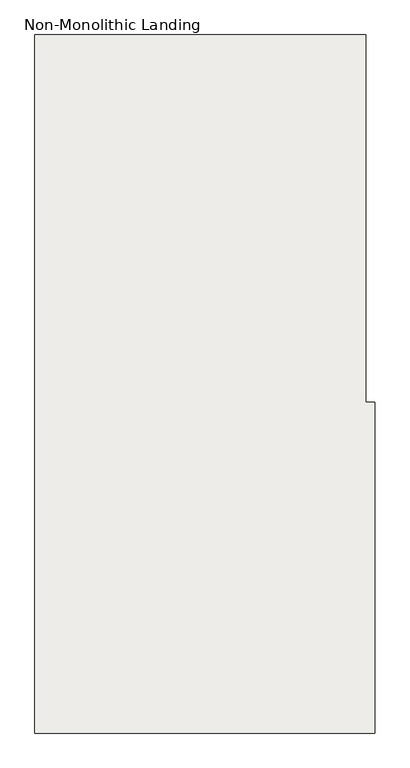
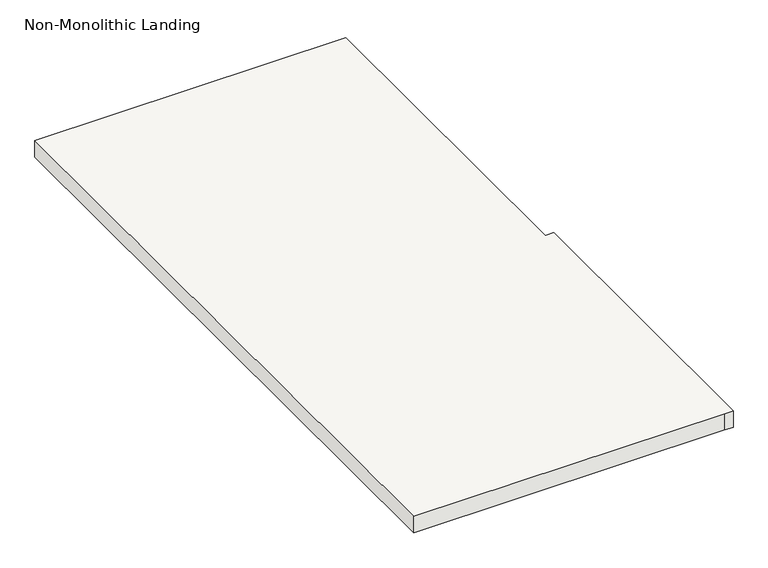
"""IFC4 building model written with IfcOpenShell, lengths in millimetres: slab geometry, Non-Monolithic Landing."""

from ifc_helpers import new_model, si_unit, origin, place, context, project, spatial, faceted_brep, source, transform, mapped, element, save


def non_monolithic_landing_c2e345a4(model_context):
    return source(origin(), model_context, "Body", "Brep", [
        faceted_brep([(-6396.9681702, -4870.057676, 1600.2), (-6396.9681702, -6800.457676, 1600.2), (-5482.5681702, -6800.457676, 1600.2), (-5457.1681702, -6800.457676, 1600.2), (-5457.1681702, -5886.057676, 1600.2), (-5482.5681702, -5886.057676, 1600.2), (-5482.5681702, -4870.057676, 1600.2), (-5507.9681702, -5784.457676, 1549.4), (-5482.5681702, -5784.457676, 1549.4), (-5482.5681702, -5886.057676, 1549.4), (-5457.1681702, -5886.057676, 1549.4), (-5457.1681702, -6800.457676, 1549.4), (-5482.5681702, -6800.457676, 1549.4), (-6396.9681702, -6800.457676, 1549.4), (-6396.9681702, -4870.057676, 1549.4), (-5507.9681702, -4870.057676, 1549.4), (-5482.5681702, -5784.457676, 1581.15), (-5482.5681702, -4870.057676, 1581.15), (-5507.9681702, -4870.057676, 1555.75), (-5507.9681702, -5784.457676, 1555.75)], [[[0, 1, 2, 3, 4, 5, 6]], [[7, 8, 9, 10, 11, 12, 13, 14, 15]], [[2, 1, 13, 12]], [[4, 3, 11, 10]], [[3, 2, 12, 11]], [[6, 5, 9, 8, 16, 17]], [[0, 6, 17, 18, 15, 14]], [[18, 17, 16, 19]], [[8, 7, 19, 16]], [[7, 15, 18, 19]], [[1, 0, 14, 13]], [[5, 4, 10, 9]]]),
    ])


if __name__ == "__main__":
    model = new_model("IFC4")
    model_context = context("Model", 3, world=origin())
    ifc_project = project(units=[si_unit("LENGTHUNIT", "METRE", prefix="MILLI")], contexts=[model_context])
    site = spatial("IfcSite", under=ifc_project)
    building = spatial("IfcBuilding", under=site)
    placement = place(None, origin())
    non_monolithic_landing_shape = non_monolithic_landing_c2e345a4(model_context)
    element("IfcSlab", 1, ObjectType="Non-Monolithic Landing", at=placement, inside=building, context=model_context, shape_type="MappedRepresentation", body=[
        mapped(non_monolithic_landing_shape, transform((0.0, 0.0, 0.0), x_axis=(1.0, 0.0, 0.0), y_axis=(0.0, 1.0, 0.0), z_axis=(0.0, 0.0, 1.0))),
    ])
    save(model, "model.ifc")
